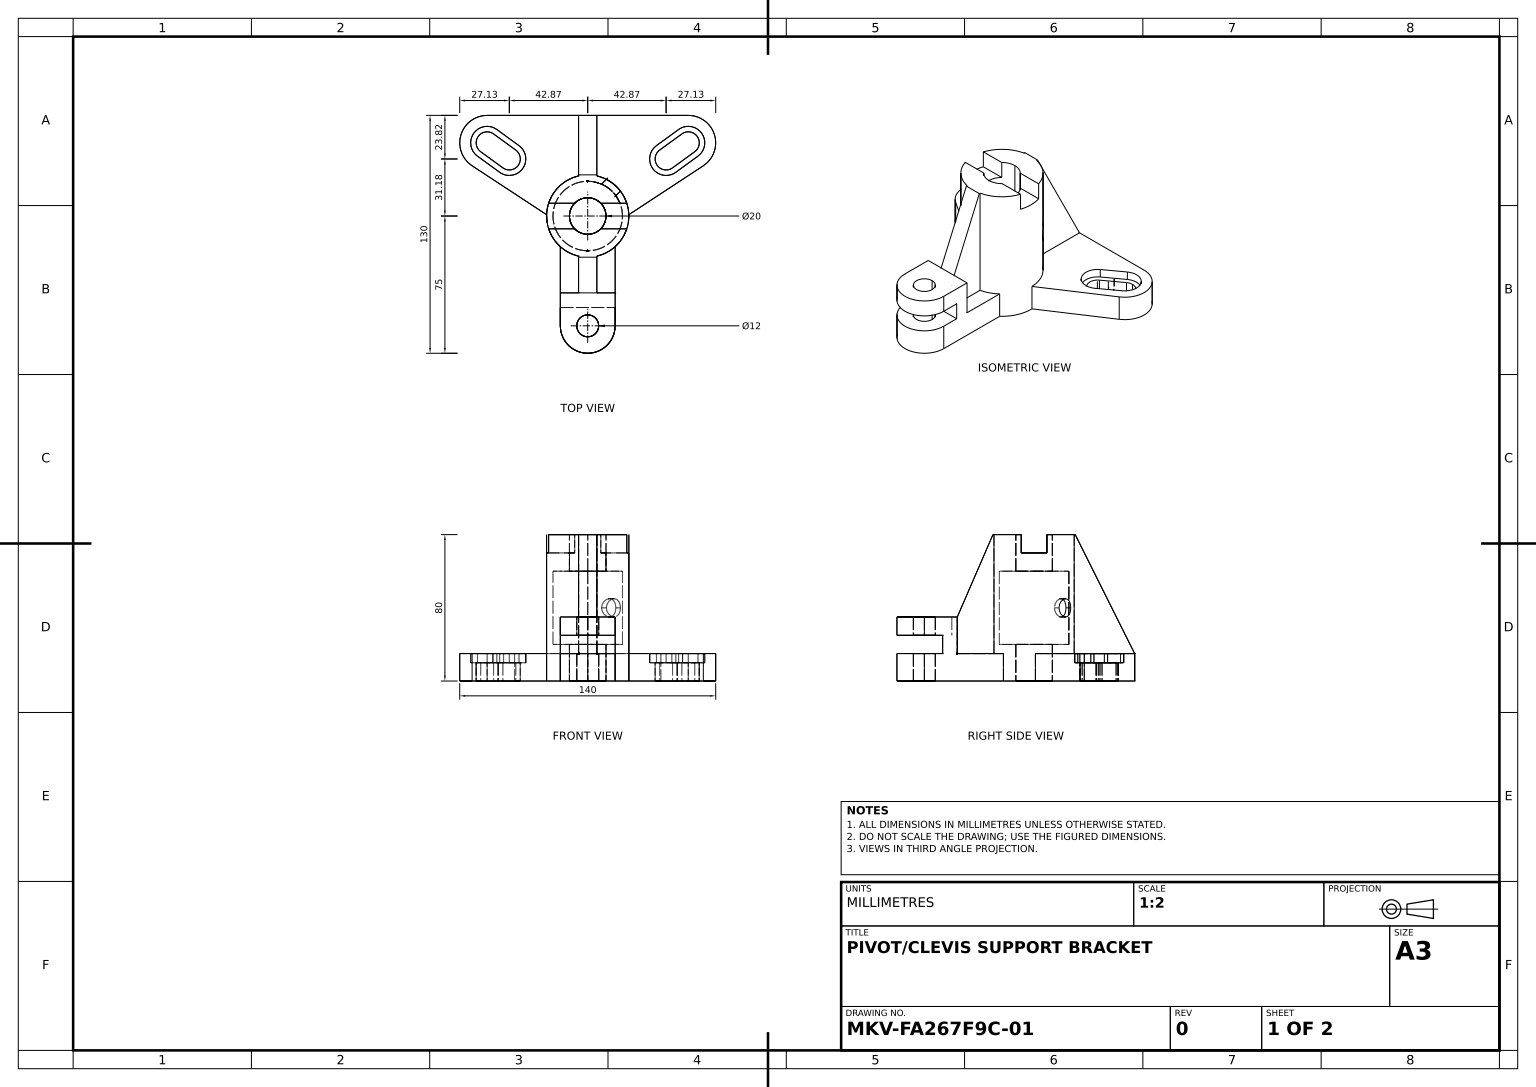
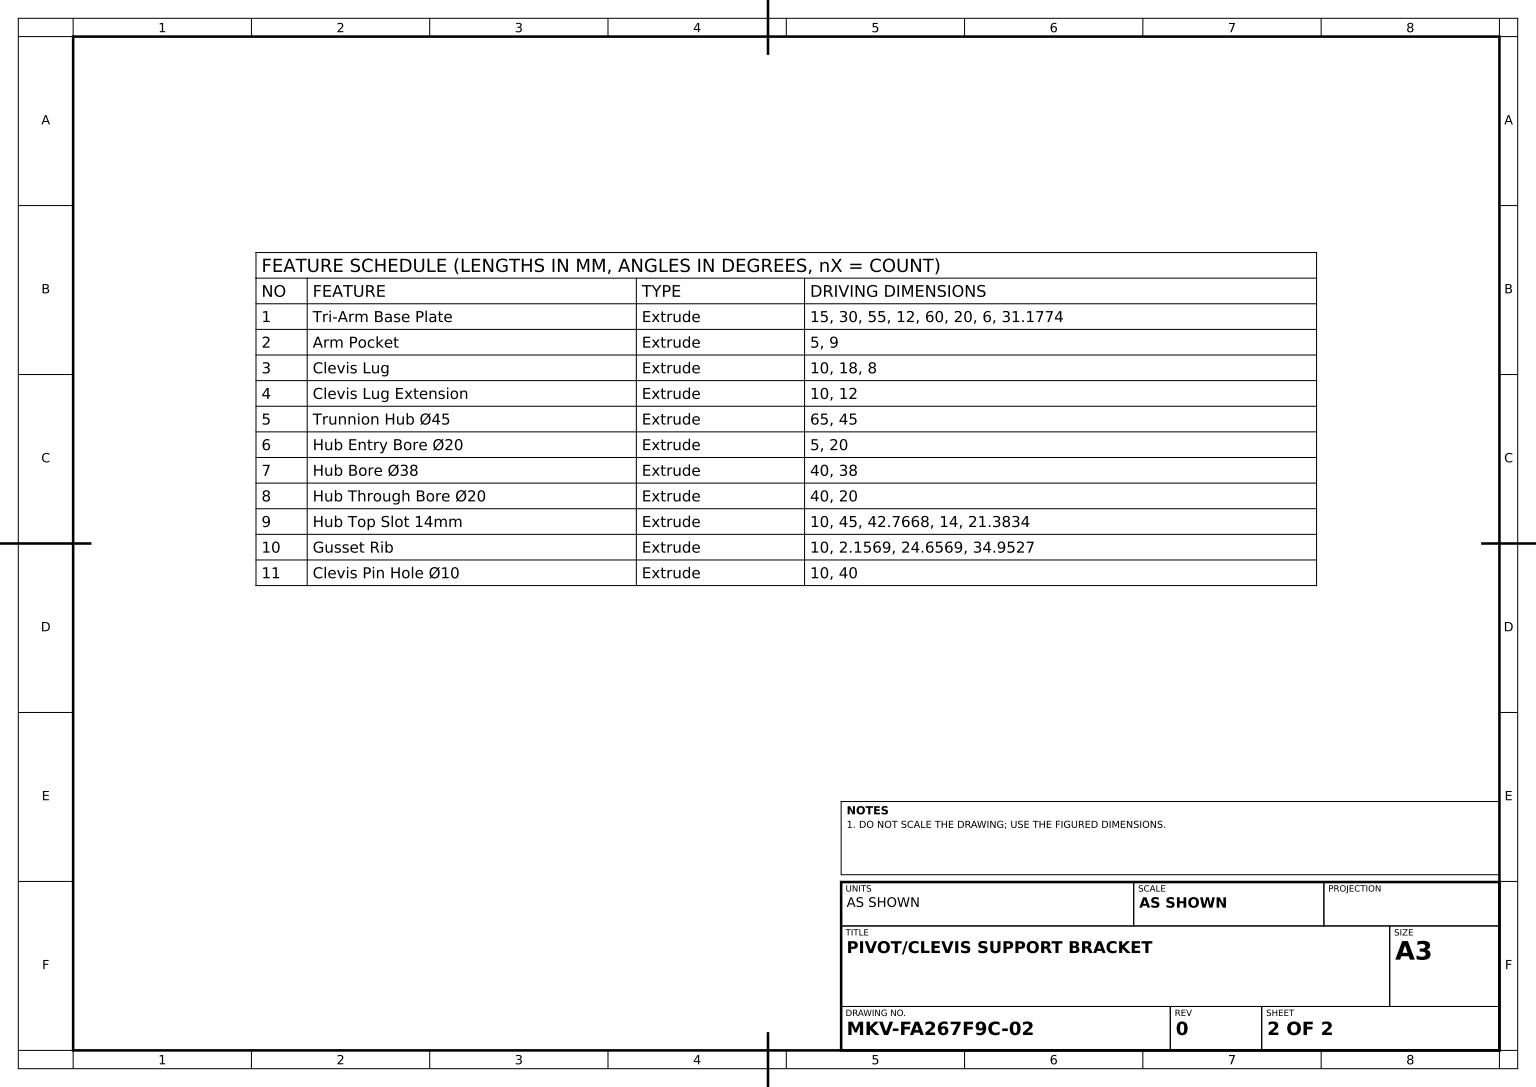
SolidWorks part; units mm, degrees
material "Plain Carbon Steel"
ref_plane "Front Plane" through (0, 0, 0) normal (0, 0, 1) x (1, 0, 0)
ref_plane "Top Plane" through (0, 0, 0) normal (0, 1, 0) x (1, 0, 0)
ref_plane "Right Plane" through (0, 0, 0) normal (1, 0, 0) x (0, 0, -1)
sketch "Tri-Arm Base Profile" plane through (0, 0, 0) normal (0, 1, 0) x (1, 0, 0)
  line L0 (-55, 55) -> (55, 55)
  line L1 (-63.2295, 27.4591) -> (-22.4883, 0.7241)
  line L2 (-15, -60) -> (-15, -16.7705)
  line L3 (22.4883, 0.7241) -> (63.2295, 27.4591)
  line L5 (15, -16.7705) -> (15, -60)
  line L7 (-55, 40) -> (-42.869, 31.1774) construction
  line L9 (-51.471, 44.8524) -> (-39.3399, 36.0298)
  line L10 (-58.529, 35.1476) -> (-46.398, 26.325)
  line L11 (55, 40) -> (42.869, 31.1774) construction
  line L12 (58.529, 35.1476) -> (46.398, 26.325)
  line L13 (51.471, 44.8524) -> (39.3399, 36.0298)
  arc A0 (-55, 55) -> (-63.2295, 27.4591) centre (-55, 40) ccw
  arc A1 (63.2295, 27.4591) -> (55, 55) centre (55, 40) ccw
  circle A2 centre (0, 0) radius 22.5
  arc A3 (-15, -60) -> (15, -60) centre (0, -60) ccw
  circle A4 centre (0, -60) radius 6
  circle A5 centre (0, 0) radius 10
  arc A6 (-51.471, 44.8524) -> (-58.529, 35.1476) centre (-55, 40) ccw
  arc A7 (-46.398, 26.325) -> (-39.3399, 36.0298) centre (-42.869, 31.1774) ccw
  arc A8 (58.529, 35.1476) -> (51.471, 44.8524) centre (55, 40) ccw
  arc A9 (39.3399, 36.0298) -> (46.398, 26.325) centre (42.869, 31.1774) ccw
  point P19 (-48.9345, 35.5887)
  point P26 (48.9345, 35.5887)
  dimension "D3" = 30
  dimension "D4" = 30
  dimension "D5" = 30
  dimension "D7" = 12
  dimension "D9" = 20
  dimension "D11" = 6
  dimension "D12" = 6
  dimension "D16" = 45
  dimension "D1" = 55
  dimension "D2" = 55
  dimension "D6" = 55
  dimension "D8" = 60
  dimension "D10" = 15
  dimension "D13" = 15
  dimension "D14" = 31.1774
  dimension "D15" = 31.1774
  dimension "D17" = 48.7299
extrude "Tri-Arm Base Plate" add sketch "Tri-Arm Base Profile" along normal blind 15 contours A2 L3 A1 L0 A0 L1 A9 L13 A8 L12 A7 L10 A6 L9 | A2 A5 | L2 A3 L5 A2 A4
sketch "Arm Pocket Profile" plane through (0, 15, 0) normal (0, 1, 0) x (1, 0, 0)
  line L0 (-55, 40) -> (-42.869, 31.1774) construction
  line L1 (-49.7065, 47.2786) -> (-37.5754, 38.456)
  line L2 (-60.2935, 32.7214) -> (-48.1625, 23.8988)
  line L3 (42.869, 31.1774) -> (55, 40) construction
  line L4 (37.5754, 38.456) -> (49.7065, 47.2786)
  line L5 (48.1625, 23.8988) -> (60.2935, 32.7214)
  arc A0 (-49.7065, 47.2786) -> (-60.2935, 32.7214) centre (-55, 40) ccw
  arc A1 (-48.1625, 23.8988) -> (-37.5754, 38.456) centre (-42.869, 31.1774) ccw
  arc A2 (37.5754, 38.456) -> (48.1625, 23.8988) centre (42.869, 31.1774) ccw
  arc A3 (60.2935, 32.7214) -> (49.7065, 47.2786) centre (55, 40) ccw
  point P4 (-48.9345, 35.5887)
  point P9 (48.9345, 35.5887)
  dimension "D1" = 9
  dimension "D2" = 9
extrude "Arm Pocket" cut sketch "Arm Pocket Profile" against normal blind 5
sketch "Clevis Lug Profile" plane through (0, 15, 0) normal (0, 1, 0) x (1, 0, 0)
  line L0 (-15, -42) -> (15, -42)
  line L1 (-15, -60) -> (-15, -16.7705) construction
  line L2 (15, -16.7705) -> (15, -60) construction
  line L4 (-15, -42) -> (15, -42)
  line L5 (-15, -42) -> (-15, -50)
  line L6 (-15, -50) -> (15, -50)
  line L7 (15, -42) -> (15, -50)
  line M13 (-15, -16.7705) -> (-15, -60)
  line M15 (15, -60) -> (15, -16.7705)
  dimension "D1" = 18
  dimension "D2" = 8
extrude "Clevis Lug" add sketch "Clevis Lug Profile" along normal blind 10 contours L6 L0 M13 M15
sketch "Clevis Lug Extension Profile" plane through (0, 25, 0) normal (0, 1, 0) x (1, 0, 0)
  line L0 (-15, -42) -> (-15, -60)
  line L1 (-15, -42) -> (15, -42)
  line L2 (15, -42) -> (15, -60)
  arc A0 (-15, -60) -> (15, -60) centre (0, -60) ccw
  circle A1 centre (0, -60) radius 6
  dimension "D1" = 12
extrude "Clevis Lug Extension" add sketch "Clevis Lug Extension Profile" along normal blind 10
sketch "Trunnion Hub Profile Ø45" plane through (0, 15, 0) normal (0, 1, 0) x (1, 0, 0)
  circle A0 centre (0, 0) radius 22.5
  dimension "D1" = 45
extrude "Trunnion Hub Ø45" add sketch "Trunnion Hub Profile Ø45" along normal blind 65
sketch "Hub Entry Bore Profile Ø20" plane through (0, 15, 0) normal (0, -1, 0) x (1, 0, 0)
  circle A0 centre (0, 0) radius 10
  dimension "D1" = 20
extrude "Hub Entry Bore Ø20" cut sketch "Hub Entry Bore Profile Ø20" against normal blind 5
sketch "Hub Bore Profile Ø38" plane through (0, 20, 0) normal (0, -1, 0) x (1, 0, 0)
  circle A0 centre (0, 0) radius 19
  dimension "D1" = 38
extrude "Hub Bore Ø38" cut sketch "Hub Bore Profile Ø38" against normal blind 40
sketch "Hub Through Bore Profile Ø20" plane through (0, 80, 0) normal (0, 1, 0) x (1, 0, 0)
  circle A0 centre (0, 0) radius 10
  dimension "D1" = 20
extrude "Hub Through Bore Ø20" cut sketch "Hub Through Bore Profile Ø20" against normal blind 40
sketch "Hub Top Slot Profile" plane through (0, 80, 0) normal (0, 1, 0) x (1, 0, 0)
  line L1 (-21.3834, -7) -> (21.3834, -7)
  line L2 (-21.3834, 7) -> (21.3834, 7)
  arc A1 (-21.3834, 7) -> (-21.3834, -7) centre (0, 0) ccw
  arc A2 (21.3834, -7) -> (21.3834, 7) centre (0, 0) ccw
  point P5 (-22.5, -7)
  point P6 (22.5, -7)
  point P7 (-22.5, 7)
  point P8 (22.5, 7)
  dimension "D3" = 45
  dimension "D1" = 42.7668
  dimension "D2" = 14
  dimension "D4" = 21.3834
extrude "Hub Top Slot 14mm" cut sketch "Hub Top Slot Profile" against normal blind 10
ref_plane "Plane1" through (0, 0, 0) normal (1, 0, 0) x (0, 0, -1)
sketch "Gusset Rib Profile" plane through (0, 0, 0) normal (1, 0, 0) x (0, 0, -1)
  line L0 (-42, 35) -> (-22.5, 80)
  line L1 (-22.5, 80) -> (-19.5, 80)
  line L2 (-7, 80) -> (-22.5, 80) construction
  line L3 (-19.5, 80) -> (-19.5, 15)
  line L4 (-16.7705, 15) -> (-42, 15) construction
  line L5 (-19.5, 15) -> (-44.1569, 15)
  line L6 (-44.1569, 15) -> (-44.1569, 35)
  line L7 (-60, 35) -> (-42, 35) construction
  line L8 (-44.1569, 35) -> (-42, 35)
  line L9 (22.5, 80) -> (55, 15)
  line L10 (55, 15) -> (20.0473, 15)
  line L11 (0.7241, 15) -> (27.4591, 15) construction
  line L12 (20.0473, 15) -> (20.0473, 80)
  line L13 (22.5, 80) -> (7, 80) construction
  line L14 (20.0473, 80) -> (22.5, 80)
  dimension "D1" = 2.1569
  dimension "D2" = 24.6569
  dimension "D3" = 34.9527
extrude "Gusset Rib" add sketch "Gusset Rib Profile" along normal mid plane 10
ref_plane "Plane2" through (0, 0, 0) normal (-0.7071, 0, 0.7071) x (0.7071, 0, 0.7071)
sketch "Clevis Pin Hole Profile Ø10" plane through (0, 0, 0) normal (-0.7071, 0, 0.7071) x (0.7071, 0, 0.7071)
  line L0 (0, 0) -> (25.6066, 0) construction
  line L1 (-11.9766, 15) -> (-11.9766, 80) construction
  circle A0 centre (-1.9766, 40) radius 5
  dimension "D1" = 10
  dimension "D2" = 40
  dimension "D3" = 10
extrude "Clevis Pin Hole Ø10" cut sketch "Clevis Pin Hole Profile Ø10" against normal through all
